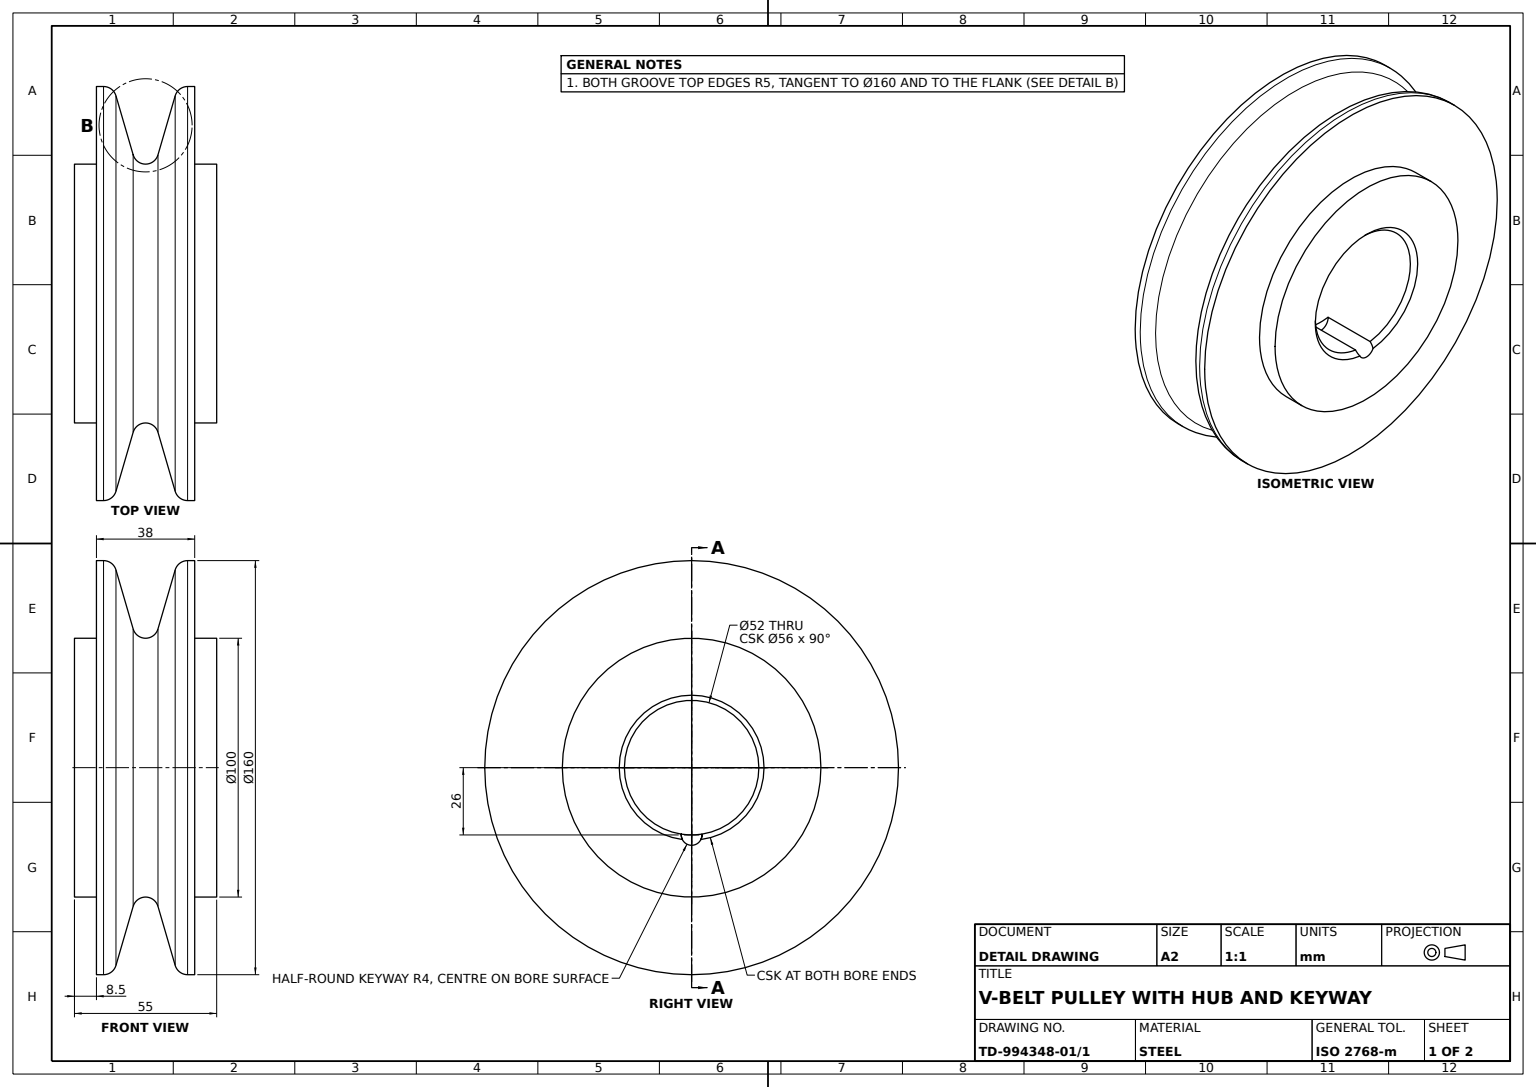
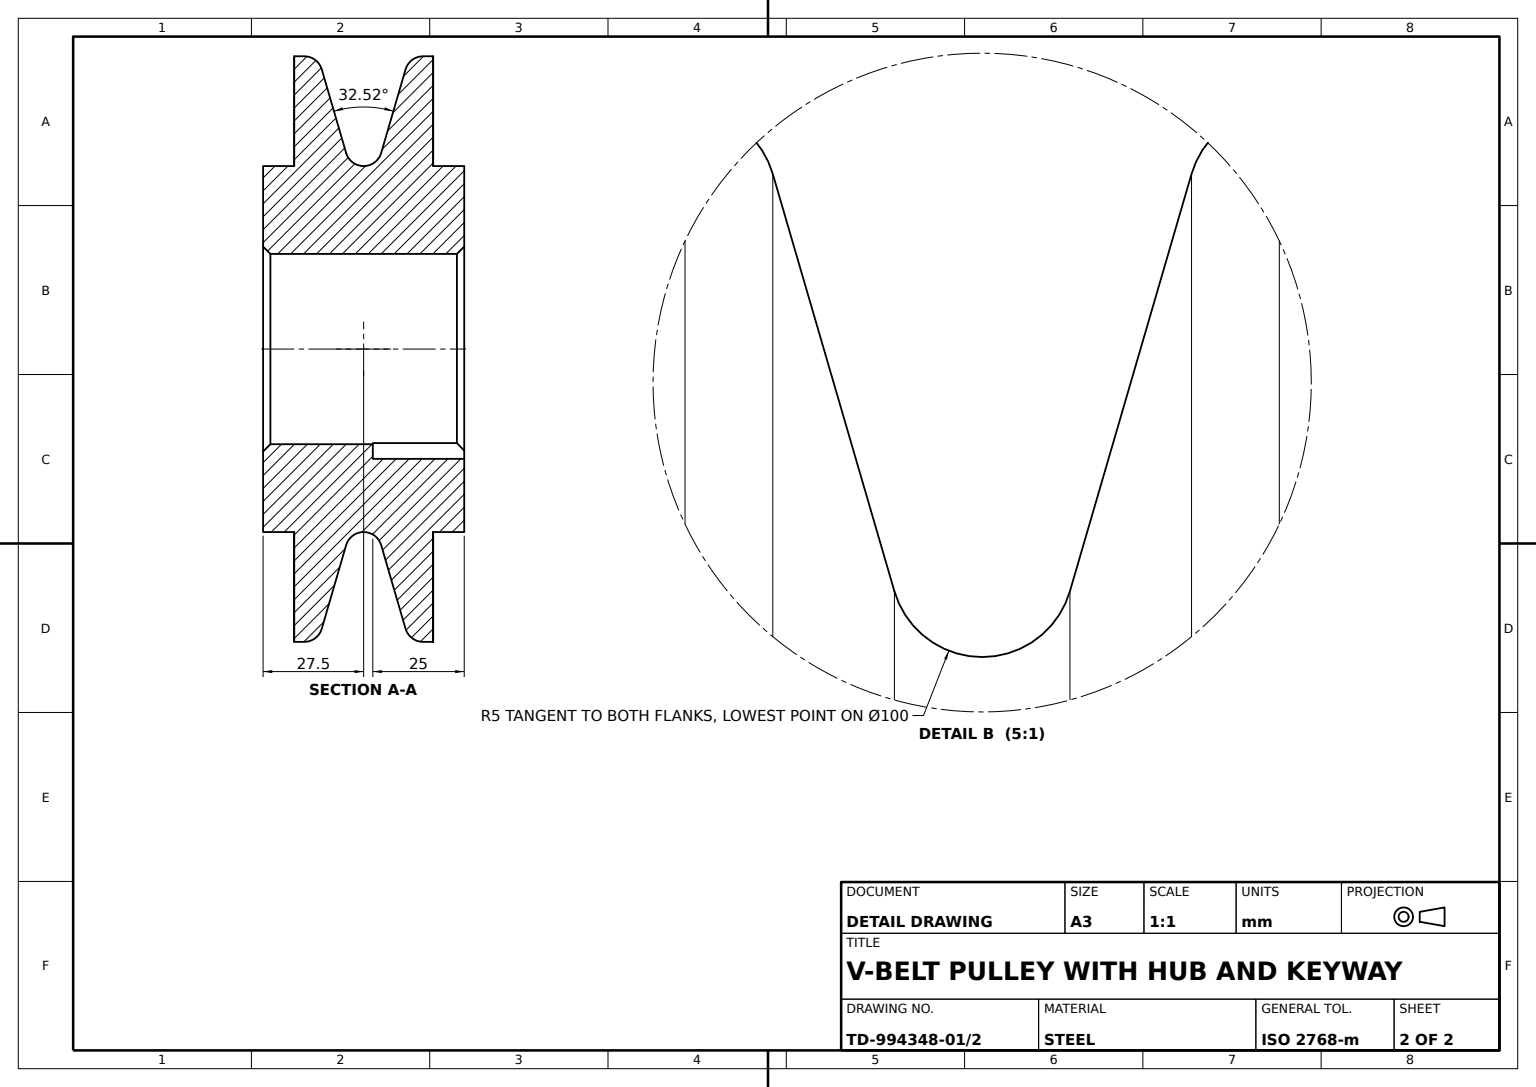
SolidWorks part; units mm, degrees
material "Plain Carbon Steel"
ref_plane "Front Plane" through (0, 0, 0) normal (0, 0, 1) x (1, 0, 0)
ref_plane "Top Plane" through (0, 0, 0) normal (0, 1, 0) x (1, 0, 0)
ref_plane "Right Plane" through (0, 0, 0) normal (1, 0, 0) x (0, 0, -1)
sketch "Pulley Profile Sketch" plane through (0, 0, 0) normal (0, 0, 1) x (1, 0, 0)
  line L0 (0, 0) -> (0, 41828.2664) construction
  line L1 (0, 0) -> (41828.2664, 0) construction
  line L2 (-27.5, 26) -> (27.5, 26)
  line L3 (27.5, 26) -> (27.5, 50)
  line L4 (27.5, 50) -> (19, 50)
  line L5 (19, 50) -> (19, 80)
  line L6 (19, 80) -> (16.25, 80)
  line L7 (11.45, 76.4) -> (4.8, 53.6)
  line L8 (-11.45, 76.4) -> (-4.8, 53.6)
  line L9 (-19, 80) -> (-16.25, 80)
  line L10 (-19, 50) -> (-19, 80)
  line L11 (-27.5, 50) -> (-19, 50)
  line L12 (-27.5, 26) -> (-27.5, 50)
  arc A0 (16.25, 80) -> (11.45, 76.4) centre (16.25, 75) ccw
  arc A1 (-11.45, 76.4) -> (-16.25, 80) centre (-16.25, 75) ccw
  arc A2 (4.8, 53.6) -> (-4.8, 53.6) centre (0, 55) cw
  point P17 (0, 26)
  point P20 (12.5, 80)
  point P23 (-12.5, 80)
  point P26 (0, 50)
  point P28 (0, 50)
  dimension "D7" = 5
  dimension "D8" = 5
  dimension "D1" = 26
  dimension "D2" = 50
  dimension "D3" = 80
  dimension "D4" = 38
  dimension "D5" = 55
  dimension "D6" = 25
revolve "Pulley Body" add sketch "Pulley Profile Sketch" angle 360 about L1
chamfer "Edge Chamfer 2mm" distance 2 angle 45 2 edges at (27.5, 0, 26) (-27.5, 0, 26)
sketch "Keyway Sketch" plane through (27.5, 0, 0) normal (1, 0, 0) x (0, 0, -1)
  circle A0 centre (0, 0) radius 26 construction
  circle A1 centre (0, 0) radius 50
  circle A2 centre (0, 0) radius 50
  circle A3 centre (0, 0) radius 26
  circle A4 centre (0, -26) radius 4
  dimension "D2" = 8
  dimension "D1" = 0
extrude "Keyway Cut 8mm" cut sketch "Keyway Sketch" against normal blind 25 contours A4
